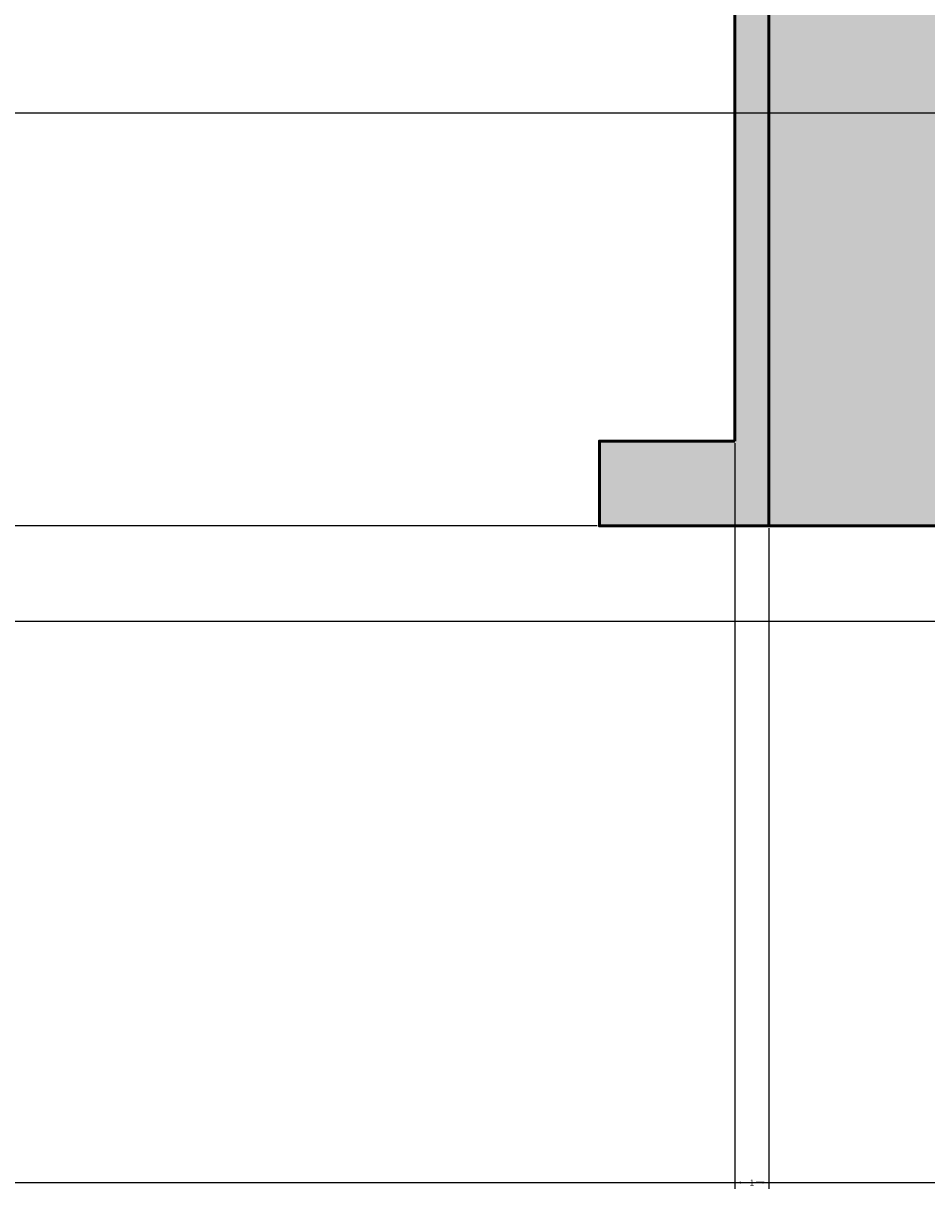
# Model space of a CAD drawing. Units: inches. Extents: x -12 to 334, y -10 to 186.
# Tile 2 of 77: x 15 to 42, y 14 to 49. Entities that reach past the tile are written whole.
import ezdxf

# ---------------------------------------------------------------- set-up
doc = ezdxf.new("R2010")
doc.units = ezdxf.units.IN
doc.header["$MEASUREMENT"] = 0
for name, color, linetype, lineweight in [('M-DIMS', 2, 'Continuous', 18), ('M-EQPM', 7, 'Continuous', 50), ('M-EQPM-PATT', 8, 'Continuous', 18)]:
    doc.layers.add(name, color=color, linetype=linetype, lineweight=lineweight)
doc.styles.get("Standard").update_dxf_attribs({"font": 'arial.ttf'})
doc.dimstyles.get("Standard").update_dxf_attribs({"dimtxt": 0.18, "dimasz": 0.18, "dimexe": 0.18, "dimexo": 0.0625, "dimgap": 0.09, "dimtad": 0, "dimtih": 1, "dimtoh": 1, "dimdec": 4, "dimzin": 0, "dimdsep": 46, "dimtxsty": 'Standard', "dimcen": 0.09, "dimadec": 0, "dimazin": 0, "dimtfac": 1, "dimtdec": 4, "dimtofl": 0, "dimtmove": 0, "dimatfit": 3, "dimfxl": 1, "dimtolj": 1, "dimtzin": 0, "dimarcsym": 0})

# ---------------------------------------------------------------- blocks, each defined once
blk = doc.blocks.new('*D1')
at = {"layer": 'Defpoints', "color": 0, "transparency": 16777216}
for p in [(281.426, 91.899), (3.376, 80.692), (281.426, 14.304)]:
    blk.add_point(p, dxfattribs=at)
at = {"layer": 'M-DIMS', "color": 0, "lineweight": -2, "transparency": 16777216}
for p, q in [((281.426, 91.836), (281.426, 14.124)), ((3.376, 80.629), (3.376, 14.124)), ((3.556, 14.304), (141.935, 14.304)), ((281.246, 14.304), (142.867, 14.304))]:
    blk.add_line(p, q, dxfattribs=at)
at = {"layer": 'M-DIMS', "color": 0, "transparency": 16777216}
for points in [[(3.556, 14.334), (3.556, 14.274), (3.376, 14.304)], [(281.246, 14.334), (281.246, 14.274), (281.426, 14.304)]]:
    blk.add_solid(points, dxfattribs=at)
at = {"layer": 'M-DIMS', "color": 0, "transparency": 16777216, "insert": (142.401, 14.304), "char_height": 0.18, "attachment_point": 5}
blk.add_mtext('\\A1;278.05', dxfattribs=at)
blk = doc.blocks.new('*D6')
at = {"layer": 'Defpoints', "color": 0, "transparency": 16777216}
for p in [(-11.174, 60.487), (23.581, 60.487), (32.1, 33.675)]:
    blk.add_point(p, dxfattribs=at)
at = {"layer": 'M-DIMS', "color": 0, "lineweight": -2, "transparency": 16777216}
for p, q in [((23.518, 60.487), (-11.354, 60.487)), ((-11.174, 60.307), (-11.174, 47.263)), ((-11.174, 33.855), (-11.174, 46.899)), ((32.038, 33.675), (-11.354, 33.675))]:
    blk.add_line(p, q, dxfattribs=at)
at = {"layer": 'M-DIMS', "color": 0, "transparency": 16777216}
for points in [[(-11.204, 60.307), (-11.144, 60.307), (-11.174, 60.487)], [(-11.204, 33.855), (-11.144, 33.855), (-11.174, 33.675)]]:
    blk.add_solid(points, dxfattribs=at)
at = {"layer": 'M-DIMS', "color": 0, "transparency": 16777216, "insert": (-11.174, 47.081), "char_height": 0.18, "attachment_point": 5}
blk.add_mtext('\\A1;26.81', dxfattribs=at)
blk = doc.blocks.new('*D9')
at = {"layer": 'Defpoints', "color": 0, "transparency": 16777216}
for p in [(36.1, 36.175), (37.1, 33.675), (37.1, 14.304)]:
    blk.add_point(p, dxfattribs=at)
at = {"layer": 'M-DIMS', "color": 0, "lineweight": -2, "transparency": 16777216}
for p, q in [((36.1, 36.113), (36.1, 14.124)), ((37.1, 33.613), (37.1, 14.124)), ((36.28, 14.304), (36.477, 14.304)), ((36.92, 14.304), (36.723, 14.304))]:
    blk.add_line(p, q, dxfattribs=at)
at = {"layer": 'M-DIMS', "color": 0, "transparency": 16777216}
for points in [[(36.28, 14.334), (36.28, 14.274), (36.1, 14.304)], [(36.92, 14.334), (36.92, 14.274), (37.1, 14.304)]]:
    blk.add_solid(points, dxfattribs=at)
at = {"layer": 'M-DIMS', "color": 0, "transparency": 16777216, "insert": (36.6, 14.304), "char_height": 0.18, "attachment_point": 5}
blk.add_mtext('\\A1;1', dxfattribs=at)
blk = doc.blocks.new('*D29')
at = {"layer": 'Defpoints', "color": 0, "transparency": 16777216}
for p in [(-11.174, 45.854), (221.576, 45.854), (216.576, 30.854)]:
    blk.add_point(p, dxfattribs=at)
at = {"layer": 'M-DIMS', "color": 0, "lineweight": -2, "transparency": 16777216}
for p, q in [((221.514, 45.854), (-11.354, 45.854)), ((-11.174, 45.674), (-11.174, 38.536)), ((-11.174, 31.034), (-11.174, 38.172)), ((216.514, 30.854), (-11.354, 30.854))]:
    blk.add_line(p, q, dxfattribs=at)
at = {"layer": 'M-DIMS', "color": 0, "transparency": 16777216}
for points in [[(-11.204, 45.674), (-11.144, 45.674), (-11.174, 45.854)], [(-11.204, 31.034), (-11.144, 31.034), (-11.174, 30.854)]]:
    blk.add_solid(points, dxfattribs=at)
at = {"layer": 'M-DIMS', "color": 0, "transparency": 16777216, "insert": (-11.174, 38.354), "char_height": 0.18, "attachment_point": 5}
blk.add_mtext('\\A1;15', dxfattribs=at)
blk = doc.blocks.new('*D39')
at = {"layer": 'Defpoints', "color": 0, "transparency": 16777216}
for p in [(279.726, 80.692), (-11.174, 45.854), (269.381, 45.854)]:
    blk.add_point(p, dxfattribs=at)
at = {"layer": 'M-DIMS', "color": 0, "lineweight": -2, "transparency": 16777216}
for p, q in [((279.664, 80.692), (-11.354, 80.692)), ((-11.174, 80.512), (-11.174, 63.455)), ((-11.174, 46.034), (-11.174, 63.091)), ((269.318, 45.854), (-11.354, 45.854))]:
    blk.add_line(p, q, dxfattribs=at)
at = {"layer": 'M-DIMS', "color": 0, "transparency": 16777216}
for points in [[(-11.204, 80.512), (-11.144, 80.512), (-11.174, 80.692)], [(-11.204, 46.034), (-11.144, 46.034), (-11.174, 45.854)]]:
    blk.add_solid(points, dxfattribs=at)
at = {"layer": 'M-DIMS', "color": 0, "transparency": 16777216, "insert": (-11.174, 63.273), "char_height": 0.18, "attachment_point": 5}
blk.add_mtext('\\A1;34.84', dxfattribs=at)

msp = doc.modelspace()

# ---------------------------------------------------------------- hatches: boundary and pattern name
at = {"layer": 'M-EQPM-PATT'}
h = msp.add_hatch(color=256, dxfattribs=at)
h.set_gradient(color1=(99, 100, 102), color2=(99, 100, 102), tint=1)
h.paths.add_polyline_path([(4.3766, 80.754, -0.4132606), (23.5807, 99.8958), (37.1002, 99.8958), (37.1002, 127.7078), (32.1002, 127.7078), (32.1002, 125.2078), (36.1002, 125.2078), (36.1002, 100.8958), (23.5807, 100.8958, 1), (23.5807, 60.4872), (36.1002, 60.4872), (36.1002, 36.1752), (32.1002, 36.1752), (32.1002, 33.6752), (37.1002, 33.6752), (37.1002, 61.4872), (23.5807, 61.4872, -0.384914), (4.4744, 78.754), (72.9244, 78.754), (72.9244, 69.6117), (75.9244, 69.6117), (75.9244, 89.8963), (72.9244, 89.8963), (72.9244, 80.754)])
h.paths.add_polyline_path([(54.1002, 125.2078), (58.1002, 125.2078), (58.1002, 127.7078), (53.1002, 127.7078), (53.1002, 99.8958), (64.5, 99.8958), (64.5, 109.0583), (63.5, 109.0583), (63.5, 100.8958), (54.1002, 100.8958)], flags=17)
h.paths.add_polyline_path([(53.1002, 33.6752), (58.1002, 33.6752), (58.1002, 36.1752), (54.1002, 36.1752), (54.1002, 60.4872), (64.2068, 60.4872), (64.2068, 49.4497), (87.8879, 49.4497), (87.8879, 55.3205), (104.8919, 55.3205), (104.8919, 30.8541), (99.8919, 30.8541), (99.8919, 28.8541), (105.8919, 28.8541), (105.8919, 56.3205), (87.8879, 56.3205), (87.8879, 63.6117), (86.8879, 63.6117), (86.8879, 50.4497), (65.0061, 50.4497), (65.0061, 63.6117), (64.5, 63.6117), (64.5, 61.4872), (53.1002, 61.4872)])
h.paths.add_polyline_path([(121.8919, 28.8541), (121.8919, 30.8541), (116.8919, 30.8541), (116.8919, 45.8541), (209.6965, 45.8541), (209.9204, 46.8541), (115.8919, 46.8541), (115.8919, 28.8541)])
h.paths.add_polyline_path([(221.5761, 32.8541), (216.5761, 32.8541), (216.5761, 30.8541), (222.5761, 30.8541), (222.5761, 46.8541), (209.9204, 46.8541), (209.6965, 45.8541), (221.5761, 45.8541)])
h.paths.add_polyline_path([(233.5761, 45.8541), (249.8485, 45.8541), (249.3759, 46.8541), (232.5761, 46.8541), (232.5761, 30.8541), (238.5761, 30.8541), (238.5761, 32.8541), (233.5761, 32.8541)])
h = msp.add_hatch(color=256, dxfattribs=at)
h.set_gradient(color1=(205, 32, 39), color2=(205, 32, 39), tint=1)
h.paths.add_polyline_path([(64.5, 80.754), (64.5, 89.8963), (226.6083, 89.8963, -1), (226.6083, 69.6117), (64.5, 69.6117), (64.5, 78.754), (4.4744, 78.754, 0.384914), (23.5807, 61.4872), (37.1002, 61.4872), (37.1002, 33.6752), (53.1002, 33.6752), (53.1002, 61.4872), (64.5, 61.4872), (64.5, 63.6117), (226.6083, 63.6117, 1), (226.6083, 95.8963), (64.5, 95.8963), (64.5, 99.8958), (53.1002, 99.8958), (53.1002, 127.7078), (37.1002, 127.7078), (37.1002, 99.8958), (23.5807, 99.8958, 0.4132606), (4.3766, 80.754)])
h.paths.add_polyline_path([(64.5, 91.8963), (64.5, 93.8963), (226.6083, 93.8963, -1), (226.6083, 65.6117), (64.5, 65.6117), (64.5, 67.6117), (226.6083, 67.6117, 1), (226.6083, 91.8963)], flags=16)

# ---------------------------------------------------------------- linework, layer by layer
at = {"layer": 'M-EQPM'}
for p, q in [((37.1002, 61.4872), (37.1002, 33.6752)), ((36.1002, 60.4872), (36.1002, 36.1752))]:
    msp.add_line(p, q, dxfattribs=at)
msp.add_lwpolyline([(36.1002, 36.1752), (32.1002, 36.1752), (32.1002, 33.6752), (58.1002, 33.6752), (58.1002, 36.1752), (54.1002, 36.1752)], dxfattribs=at)

# ---------------------------------------------------------------- dimensions: what is measured, and where the dimension line sits
at = {"layer": 'M-DIMS'}
for base, p1, p2, override, picture, middle in [((281.4256, 14.3041), (3.3765, 80.6915), (281.4256, 91.8988), {"dimdec": 2, "dimlfac": 1, "dimrnd": 0, "dimzin": 0, "dimdsep": 46, "dimlunit": 2}, '*D1', (142.401, 14.3041)), ((37.1002, 14.3041), (36.1002, 36.1752), (37.1002, 33.6752), {"dimdec": 0, "dimlfac": 1, "dimrnd": 0, "dimzin": 0, "dimdsep": 46, "dimlunit": 2}, '*D9', (36.6002, 14.3041))]:
    dim = msp.add_linear_dim(base=base, p1=p1, p2=p2, dimstyle='Standard', override=override, dxfattribs=at)
    dim.commit()
    dim.dimension.update_dxf_attribs({"geometry": picture, "text_midpoint": middle})
for base, p1, p2, override, picture, middle in [((-11.1736, 45.8541), (279.7263, 80.6915), (269.3808, 45.8541), {"dimdec": 2, "dimlfac": 1, "dimrnd": 0, "dimzin": 0, "dimdsep": 46, "dimlunit": 2}, '*D39', (-11.1735, 63.2728)), ((-11.1736, 60.4872), (32.1002, 33.6752), (23.5807, 60.4872), {"dimdec": 2, "dimlfac": 1, "dimrnd": 0, "dimzin": 0, "dimdsep": 46, "dimlunit": 2}, '*D6', (-11.1735, 47.0812)), ((-11.1736, 45.8541), (216.5761, 30.8541), (221.5761, 45.8541), {"dimdec": 0, "dimlfac": 1, "dimrnd": 0, "dimzin": 0, "dimdsep": 46, "dimlunit": 2}, '*D29', (-11.1735, 38.3541))]:
    dim = msp.add_linear_dim(base=base, p1=p1, p2=p2, angle=90, dimstyle='Standard', override=override, dxfattribs=at)
    dim.commit()
    dim.dimension.update_dxf_attribs({"geometry": picture, "text_midpoint": middle})

doc.saveas('drawing.dxf')
